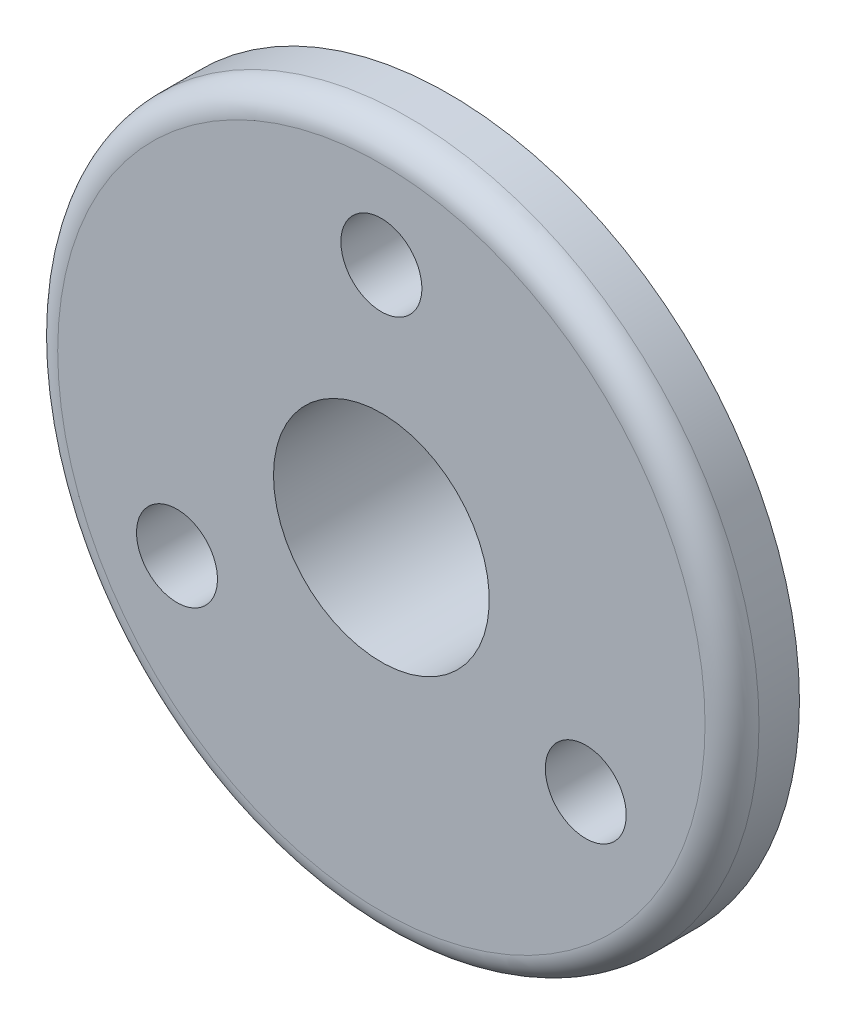
ISO-10303-21;
HEADER;
FILE_DESCRIPTION(('STEP AP214'),'2;1');
FILE_NAME('part.step','',(''),(''),'','','');
FILE_SCHEMA(('AUTOMOTIVE_DESIGN { 1 0 10303 214 1 1 1 1 }'));
ENDSEC;
DATA;
#1=APPLICATION_CONTEXT('core data for automotive mechanical design processes');
#2=APPLICATION_PROTOCOL_DEFINITION('international standard','automotive_design',2000,#1);
#3=PRODUCT_CONTEXT('',#1,'mechanical');
#4=PRODUCT('Part','Part','',(#3));
#5=PRODUCT_RELATED_PRODUCT_CATEGORY('part','',(#4));
#6=PRODUCT_DEFINITION_FORMATION('','',#4);
#7=PRODUCT_DEFINITION_CONTEXT('part definition',#1,'design');
#8=PRODUCT_DEFINITION('design','',#6,#7);
#9=PRODUCT_DEFINITION_SHAPE('','',#8);
#10=(LENGTH_UNIT() NAMED_UNIT(*) SI_UNIT(.MILLI.,.METRE.));
#11=(NAMED_UNIT(*) PLANE_ANGLE_UNIT() SI_UNIT($,.RADIAN.));
#12=(NAMED_UNIT(*) SI_UNIT($,.STERADIAN.) SOLID_ANGLE_UNIT());
#13=UNCERTAINTY_MEASURE_WITH_UNIT(LENGTH_MEASURE(1.E-05),#10,'distance_accuracy_value','');
#14=(GEOMETRIC_REPRESENTATION_CONTEXT(3) GLOBAL_UNCERTAINTY_ASSIGNED_CONTEXT((#13)) GLOBAL_UNIT_ASSIGNED_CONTEXT((#10,
#11,#12)) REPRESENTATION_CONTEXT('',''));
#15=CARTESIAN_POINT('',(0.,0.,0.));
#16=DIRECTION('',(0.,0.,1.));
#17=DIRECTION('',(1.,0.,0.));
#18=AXIS2_PLACEMENT_3D('',#15,#16,#17);
#19=CARTESIAN_POINT('',(0.,0.,-5.));
#20=DIRECTION('',(0.,0.,1.));
#21=DIRECTION('',(1.,0.,0.));
#22=AXIS2_PLACEMENT_3D('',#19,#20,#21);
#23=CYLINDRICAL_SURFACE('',#22,26.);
#24=CARTESIAN_POINT('',(0.,0.,-2.));
#25=DIRECTION('',(0.,0.,1.));
#26=DIRECTION('',(1.,0.,0.));
#27=AXIS2_PLACEMENT_3D('',#24,#25,#26);
#28=CIRCLE('',#27,26.);
#29=CARTESIAN_POINT('',(26.,0.,-2.));
#30=VERTEX_POINT('',#29);
#31=EDGE_CURVE('E10',#30,#30,#28,.F.);
#32=ORIENTED_EDGE('',*,*,#31,.T.);
#33=EDGE_LOOP('',(#32));
#34=FACE_BOUND('',#33,.T.);
#35=CARTESIAN_POINT('',(0.,0.,-5.));
#36=DIRECTION('',(0.,0.,1.));
#37=DIRECTION('',(1.,0.,0.));
#38=AXIS2_PLACEMENT_3D('',#35,#36,#37);
#39=CIRCLE('',#38,26.);
#40=CARTESIAN_POINT('',(26.,0.,-5.));
#41=VERTEX_POINT('',#40);
#42=EDGE_CURVE('E59',#41,#41,#39,.T.);
#43=ORIENTED_EDGE('',*,*,#42,.T.);
#44=EDGE_LOOP('',(#43));
#45=FACE_BOUND('',#44,.T.);
#46=ADVANCED_FACE('F43',(#34,#45),#23,.T.);
#47=CARTESIAN_POINT('',(0.,0.,-5.));
#48=DIRECTION('',(0.,0.,1.));
#49=DIRECTION('',(1.,0.,0.));
#50=AXIS2_PLACEMENT_3D('',#47,#48,#49);
#51=PLANE('',#50);
#52=CARTESIAN_POINT('',(0.,17.5,-5.));
#53=DIRECTION('',(0.,0.,-1.));
#54=DIRECTION('',(-1.,0.,0.));
#55=AXIS2_PLACEMENT_3D('',#52,#53,#54);
#56=CIRCLE('',#55,3.);
#57=CARTESIAN_POINT('',(-3.,17.5,-5.));
#58=VERTEX_POINT('',#57);
#59=EDGE_CURVE('E82',#58,#58,#56,.T.);
#60=ORIENTED_EDGE('',*,*,#59,.F.);
#61=EDGE_LOOP('',(#60));
#62=FACE_BOUND('',#61,.T.);
#63=CARTESIAN_POINT('',(-15.1554445662277,-8.75,-5.));
#64=DIRECTION('',(0.,0.,-1.));
#65=DIRECTION('',(-1.,0.,0.));
#66=AXIS2_PLACEMENT_3D('',#63,#64,#65);
#67=CIRCLE('',#66,3.00000000000008);
#68=CARTESIAN_POINT('',(-18.1554445662278,-8.75,-5.));
#69=VERTEX_POINT('',#68);
#70=EDGE_CURVE('E81',#69,#69,#67,.T.);
#71=ORIENTED_EDGE('',*,*,#70,.F.);
#72=EDGE_LOOP('',(#71));
#73=FACE_BOUND('',#72,.T.);
#74=CARTESIAN_POINT('',(15.1554445662277,-8.75000000000001,-5.));
#75=DIRECTION('',(0.,0.,-1.));
#76=DIRECTION('',(-1.,0.,0.));
#77=AXIS2_PLACEMENT_3D('',#74,#75,#76);
#78=CIRCLE('',#77,3.00000000000016);
#79=CARTESIAN_POINT('',(12.1554445662275,-8.75000000000001,-5.));
#80=VERTEX_POINT('',#79);
#81=EDGE_CURVE('E77',#80,#80,#78,.T.);
#82=ORIENTED_EDGE('',*,*,#81,.F.);
#83=EDGE_LOOP('',(#82));
#84=FACE_BOUND('',#83,.T.);
#85=CARTESIAN_POINT('',(0.,0.,-5.));
#86=DIRECTION('',(0.,0.,-1.));
#87=DIRECTION('',(-1.,0.,0.));
#88=AXIS2_PLACEMENT_3D('',#85,#86,#87);
#89=CIRCLE('',#88,12.5);
#90=CARTESIAN_POINT('',(-12.5,0.,-5.));
#91=VERTEX_POINT('',#90);
#92=EDGE_CURVE('E53',#91,#91,#89,.T.);
#93=ORIENTED_EDGE('',*,*,#92,.F.);
#94=EDGE_LOOP('',(#93));
#95=FACE_BOUND('',#94,.T.);
#96=ORIENTED_EDGE('',*,*,#42,.F.);
#97=EDGE_LOOP('',(#96));
#98=FACE_BOUND('',#97,.T.);
#99=ADVANCED_FACE('F103',(#62,#73,#84,#95,#98),#51,.F.);
#100=CARTESIAN_POINT('',(0.,0.,0.));
#101=DIRECTION('',(0.,0.,1.));
#102=DIRECTION('',(1.,0.,0.));
#103=AXIS2_PLACEMENT_3D('',#100,#101,#102);
#104=PLANE('',#103);
#105=CARTESIAN_POINT('',(0.,0.,0.));
#106=DIRECTION('',(0.,0.,1.));
#107=DIRECTION('',(1.,0.,0.));
#108=AXIS2_PLACEMENT_3D('',#105,#106,#107);
#109=CIRCLE('',#108,24.);
#110=CARTESIAN_POINT('',(24.,0.,0.));
#111=VERTEX_POINT('',#110);
#112=EDGE_CURVE('E49',#111,#111,#109,.T.);
#113=ORIENTED_EDGE('',*,*,#112,.T.);
#114=EDGE_LOOP('',(#113));
#115=FACE_BOUND('',#114,.T.);
#116=CARTESIAN_POINT('',(0.,17.5,0.));
#117=DIRECTION('',(0.,0.,-1.));
#118=DIRECTION('',(-1.,0.,0.));
#119=AXIS2_PLACEMENT_3D('',#116,#117,#118);
#120=CIRCLE('',#119,3.);
#121=CARTESIAN_POINT('',(-3.,17.5,0.));
#122=VERTEX_POINT('',#121);
#123=EDGE_CURVE('E66',#122,#122,#120,.T.);
#124=ORIENTED_EDGE('',*,*,#123,.T.);
#125=EDGE_LOOP('',(#124));
#126=FACE_BOUND('',#125,.T.);
#127=CARTESIAN_POINT('',(-15.1554445662277,-8.75,0.));
#128=DIRECTION('',(0.,0.,-1.));
#129=DIRECTION('',(-1.,0.,0.));
#130=AXIS2_PLACEMENT_3D('',#127,#128,#129);
#131=CIRCLE('',#130,3.00000000000008);
#132=CARTESIAN_POINT('',(-18.1554445662278,-8.75,0.));
#133=VERTEX_POINT('',#132);
#134=EDGE_CURVE('E79',#133,#133,#131,.T.);
#135=ORIENTED_EDGE('',*,*,#134,.T.);
#136=EDGE_LOOP('',(#135));
#137=FACE_BOUND('',#136,.T.);
#138=CARTESIAN_POINT('',(15.1554445662277,-8.75000000000001,0.));
#139=DIRECTION('',(0.,0.,-1.));
#140=DIRECTION('',(-1.,0.,0.));
#141=AXIS2_PLACEMENT_3D('',#138,#139,#140);
#142=CIRCLE('',#141,3.00000000000016);
#143=CARTESIAN_POINT('',(12.1554445662275,-8.75000000000001,0.));
#144=VERTEX_POINT('',#143);
#145=EDGE_CURVE('E72',#144,#144,#142,.T.);
#146=ORIENTED_EDGE('',*,*,#145,.T.);
#147=EDGE_LOOP('',(#146));
#148=FACE_BOUND('',#147,.T.);
#149=CARTESIAN_POINT('',(0.,0.,0.));
#150=DIRECTION('',(0.,0.,-1.));
#151=DIRECTION('',(-1.,0.,0.));
#152=AXIS2_PLACEMENT_3D('',#149,#150,#151);
#153=CIRCLE('',#152,8.);
#154=CARTESIAN_POINT('',(-8.,0.,0.));
#155=VERTEX_POINT('',#154);
#156=EDGE_CURVE('E67',#155,#155,#153,.T.);
#157=ORIENTED_EDGE('',*,*,#156,.T.);
#158=EDGE_LOOP('',(#157));
#159=FACE_BOUND('',#158,.T.);
#160=ADVANCED_FACE('F91',(#115,#126,#137,#148,#159),#104,.T.);
#161=CARTESIAN_POINT('',(0.,0.,-12.));
#162=DIRECTION('',(0.,0.,1.));
#163=DIRECTION('',(1.,0.,0.));
#164=AXIS2_PLACEMENT_3D('',#161,#162,#163);
#165=CYLINDRICAL_SURFACE('',#164,12.5);
#166=CARTESIAN_POINT('',(0.,0.,-12.));
#167=DIRECTION('',(0.,0.,-1.));
#168=DIRECTION('',(-1.,0.,0.));
#169=AXIS2_PLACEMENT_3D('',#166,#167,#168);
#170=CIRCLE('',#169,12.5);
#171=CARTESIAN_POINT('',(-12.5,0.,-12.));
#172=VERTEX_POINT('',#171);
#173=EDGE_CURVE('E61',#172,#172,#170,.T.);
#174=ORIENTED_EDGE('',*,*,#173,.F.);
#175=EDGE_LOOP('',(#174));
#176=FACE_BOUND('',#175,.T.);
#177=ORIENTED_EDGE('',*,*,#92,.T.);
#178=EDGE_LOOP('',(#177));
#179=FACE_BOUND('',#178,.T.);
#180=ADVANCED_FACE('F118',(#176,#179),#165,.T.);
#181=CARTESIAN_POINT('',(0.,0.,-12.));
#182=DIRECTION('',(0.,0.,-1.));
#183=DIRECTION('',(-1.,0.,0.));
#184=AXIS2_PLACEMENT_3D('',#181,#182,#183);
#185=PLANE('',#184);
#186=CARTESIAN_POINT('',(0.,0.,-12.));
#187=DIRECTION('',(0.,0.,-1.));
#188=DIRECTION('',(-1.,0.,0.));
#189=AXIS2_PLACEMENT_3D('',#186,#187,#188);
#190=CIRCLE('',#189,8.);
#191=CARTESIAN_POINT('',(-8.,0.,-12.));
#192=VERTEX_POINT('',#191);
#193=EDGE_CURVE('E70',#192,#192,#190,.T.);
#194=ORIENTED_EDGE('',*,*,#193,.F.);
#195=EDGE_LOOP('',(#194));
#196=FACE_BOUND('',#195,.T.);
#197=ORIENTED_EDGE('',*,*,#173,.T.);
#198=EDGE_LOOP('',(#197));
#199=FACE_BOUND('',#198,.T.);
#200=ADVANCED_FACE('F124',(#196,#199),#185,.T.);
#201=CARTESIAN_POINT('',(0.,0.,0.));
#202=DIRECTION('',(0.,0.,-1.));
#203=DIRECTION('',(-1.,0.,0.));
#204=AXIS2_PLACEMENT_3D('',#201,#202,#203);
#205=CYLINDRICAL_SURFACE('',#204,8.);
#206=ORIENTED_EDGE('',*,*,#156,.F.);
#207=EDGE_LOOP('',(#206));
#208=FACE_BOUND('',#207,.T.);
#209=ORIENTED_EDGE('',*,*,#193,.T.);
#210=EDGE_LOOP('',(#209));
#211=FACE_BOUND('',#210,.T.);
#212=ADVANCED_FACE('F126',(#208,#211),#205,.F.);
#213=CARTESIAN_POINT('',(15.1554445662277,-8.75000000000001,0.));
#214=DIRECTION('',(0.,0.,-1.));
#215=DIRECTION('',(-1.,0.,0.));
#216=AXIS2_PLACEMENT_3D('',#213,#214,#215);
#217=CYLINDRICAL_SURFACE('',#216,3.00000000000016);
#218=ORIENTED_EDGE('',*,*,#145,.F.);
#219=EDGE_LOOP('',(#218));
#220=FACE_BOUND('',#219,.T.);
#221=ORIENTED_EDGE('',*,*,#81,.T.);
#222=EDGE_LOOP('',(#221));
#223=FACE_BOUND('',#222,.T.);
#224=ADVANCED_FACE('F132',(#220,#223),#217,.F.);
#225=CARTESIAN_POINT('',(-15.1554445662277,-8.75,0.));
#226=DIRECTION('',(0.,0.,-1.));
#227=DIRECTION('',(-1.,0.,0.));
#228=AXIS2_PLACEMENT_3D('',#225,#226,#227);
#229=CYLINDRICAL_SURFACE('',#228,3.00000000000008);
#230=ORIENTED_EDGE('',*,*,#134,.F.);
#231=EDGE_LOOP('',(#230));
#232=FACE_BOUND('',#231,.T.);
#233=ORIENTED_EDGE('',*,*,#70,.T.);
#234=EDGE_LOOP('',(#233));
#235=FACE_BOUND('',#234,.T.);
#236=ADVANCED_FACE('F97',(#232,#235),#229,.F.);
#237=CARTESIAN_POINT('',(0.,17.5,0.));
#238=DIRECTION('',(0.,0.,-1.));
#239=DIRECTION('',(-1.,0.,0.));
#240=AXIS2_PLACEMENT_3D('',#237,#238,#239);
#241=CYLINDRICAL_SURFACE('',#240,3.);
#242=ORIENTED_EDGE('',*,*,#123,.F.);
#243=EDGE_LOOP('',(#242));
#244=FACE_BOUND('',#243,.T.);
#245=ORIENTED_EDGE('',*,*,#59,.T.);
#246=EDGE_LOOP('',(#245));
#247=FACE_BOUND('',#246,.T.);
#248=ADVANCED_FACE('F93',(#244,#247),#241,.F.);
#249=CARTESIAN_POINT('',(0.,0.,-2.));
#250=DIRECTION('',(0.,0.,1.));
#251=DIRECTION('',(1.,0.,0.));
#252=AXIS2_PLACEMENT_3D('',#249,#250,#251);
#253=TOROIDAL_SURFACE('',#252,24.,2.);
#254=ORIENTED_EDGE('',*,*,#31,.F.);
#255=EDGE_LOOP('',(#254));
#256=FACE_BOUND('',#255,.T.);
#257=ORIENTED_EDGE('',*,*,#112,.F.);
#258=EDGE_LOOP('',(#257));
#259=FACE_BOUND('',#258,.T.);
#260=ADVANCED_FACE('F44',(#256,#259),#253,.T.);
#261=CLOSED_SHELL('',(#46,#99,#160,#180,#200,#212,#224,#236,#248,#260));
#262=MANIFOLD_SOLID_BREP('B2',#261);
#263=ADVANCED_BREP_SHAPE_REPRESENTATION('',(#18,#262),#14);
#264=SHAPE_DEFINITION_REPRESENTATION(#9,#263);
ENDSEC;
END-ISO-10303-21;
